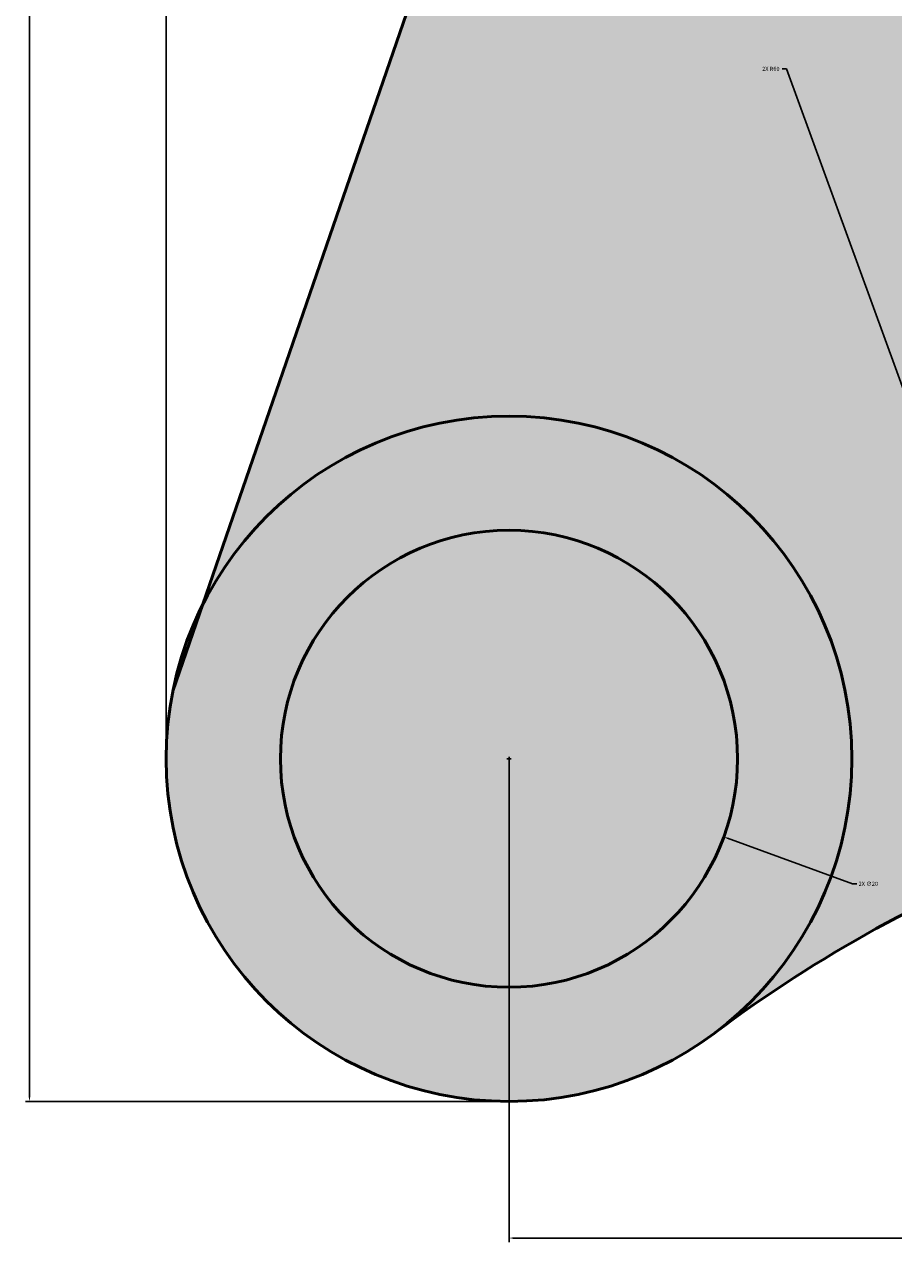
# Model space of a CAD drawing. Units: inches. Extents: x 114 to 236, y -51 to 115.
# Tile 2 of 14: x 114 to 152, y -13 to 41. Entities that reach past the tile are written whole.
import ezdxf

# ---------------------------------------------------------------- set-up
doc = ezdxf.new("R2010")
doc.units = ezdxf.units.IN
doc.header["$MEASUREMENT"] = 0
doc.layers.add('M-DIMS', color=2, linetype='Continuous', lineweight=18)
doc.layers.add('M-OUTL', color=7, linetype='Continuous', lineweight=50)
doc.layers.add('M-HATC', color=7, linetype='Continuous', lineweight=18, true_color=0xffffff)
doc.styles.get("Standard").update_dxf_attribs({"font": 'arial.ttf'})
doc.dimstyles.get("Standard").update_dxf_attribs({"dimtxt": 0.18, "dimasz": 0.18, "dimexe": 0.18, "dimexo": 0.0625, "dimgap": 0.09, "dimtad": 0, "dimtih": 1, "dimtoh": 1, "dimdec": 4, "dimzin": 0, "dimdsep": 46, "dimtxsty": 'Standard', "dimcen": 0.09, "dimadec": 0, "dimazin": 0, "dimtfac": 1, "dimtdec": 4, "dimtofl": 0, "dimtmove": 0, "dimatfit": 3, "dimfxl": 1, "dimtolj": 1, "dimtzin": 0, "dimarcsym": 0})

# ---------------------------------------------------------------- blocks, each defined once
blk = doc.blocks.new('BOSS-OD30-ID20')
for radius in [15, 10]:
    blk.add_circle((0, 0), radius)
blk = doc.blocks.new('*D3')
at = {"layer": 'Defpoints', "color": 0, "transparency": 16777216}
for p in [(230.229, 115.287), (120.229, 9.307), (230.229, 9.307)]:
    blk.add_point(p, dxfattribs=at)
at = {"layer": 'M-DIMS', "color": 0, "lineweight": -2, "transparency": 16777216}
for p, q in [((120.229, 9.37), (120.229, 115.467)), ((120.409, 115.287), (174.949, 115.287)), ((230.049, 115.287), (175.509, 115.287)), ((230.229, 9.37), (230.229, 115.467))]:
    blk.add_line(p, q, dxfattribs=at)
at = {"layer": 'M-DIMS', "color": 0, "transparency": 16777216}
for points in [[(120.409, 115.317), (120.409, 115.257), (120.229, 115.287)], [(230.049, 115.317), (230.049, 115.257), (230.229, 115.287)]]:
    blk.add_solid(points, dxfattribs=at)
at = {"layer": 'M-DIMS', "color": 0, "transparency": 16777216, "insert": (175.229, 115.287), "char_height": 0.18, "attachment_point": 5}
blk.add_mtext('\\A1;110', dxfattribs=at)
blk = doc.blocks.new('*D4')
at = {"layer": 'Defpoints', "color": 0, "transparency": 16777216}
for p in [(114.249, 109.307), (175.229, 109.307), (135.229, -5.693)]:
    blk.add_point(p, dxfattribs=at)
at = {"layer": 'M-DIMS', "color": 0, "lineweight": -2, "transparency": 16777216}
for p, q in [((175.166, 109.307), (114.069, 109.307)), ((114.249, 109.127), (114.249, 51.989)), ((114.249, -5.513), (114.249, 51.625)), ((135.166, -5.693), (114.069, -5.693))]:
    blk.add_line(p, q, dxfattribs=at)
at = {"layer": 'M-DIMS', "color": 0, "transparency": 16777216}
for points in [[(114.219, 109.127), (114.279, 109.127), (114.249, 109.307)], [(114.219, -5.513), (114.279, -5.513), (114.249, -5.693)]]:
    blk.add_solid(points, dxfattribs=at)
at = {"layer": 'M-DIMS', "color": 0, "transparency": 16777216, "insert": (114.249, 51.807), "char_height": 0.18, "attachment_point": 5}
blk.add_mtext('\\A1;115', dxfattribs=at)
blk = doc.blocks.new('*D5')
at = {"layer": 'Defpoints', "color": 0, "transparency": 16777216}
for p in [(175.229, 79.307), (135.229, 9.307), (175.229, -11.673)]:
    blk.add_point(p, dxfattribs=at)
at = {"layer": 'M-DIMS', "color": 0, "lineweight": -2, "transparency": 16777216}
for p, q in [((175.229, 79.245), (175.229, -11.853)), ((135.229, 9.245), (135.229, -11.853)), ((135.409, -11.673), (155.006, -11.673)), ((175.049, -11.673), (155.451, -11.673))]:
    blk.add_line(p, q, dxfattribs=at)
at = {"layer": 'M-DIMS', "color": 0, "transparency": 16777216}
for points in [[(135.409, -11.643), (135.409, -11.703), (135.229, -11.673)], [(175.049, -11.643), (175.049, -11.703), (175.229, -11.673)]]:
    blk.add_solid(points, dxfattribs=at)
at = {"layer": 'M-DIMS', "color": 0, "transparency": 16777216, "insert": (155.229, -11.673), "char_height": 0.18, "attachment_point": 5}
blk.add_mtext('\\A1;40', dxfattribs=at)
blk = doc.blocks.new('*D13')
at = {"layer": 'Defpoints', "color": 0, "transparency": 16777216}
for p in [(125.832, 12.727), (144.626, 5.887)]:
    blk.add_point(p, dxfattribs=at)
at = {"layer": 'M-DIMS', "color": 0, "lineweight": -2, "transparency": 16777216}
for p, q in [((135.139, 9.307), (135.319, 9.307)), ((135.229, 9.217), (135.229, 9.397)), ((150.264, 3.835), (144.795, 5.825)), ((150.444, 3.835), (150.264, 3.835))]:
    blk.add_line(p, q, dxfattribs=at)
at = {"layer": 'M-DIMS', "color": 0, "transparency": 16777216}
blk.add_solid([(144.805, 5.853), (144.784, 5.797), (144.626, 5.887)], dxfattribs=at)
at = {"layer": 'M-DIMS', "color": 0, "transparency": 16777216, "insert": (150.95, 3.835), "char_height": 0.18, "attachment_point": 5}
blk.add_mtext('\\A1;2X ∅20', dxfattribs=at)
blk = doc.blocks.new('*D14')
at = {"layer": 'Defpoints', "color": 0, "transparency": 16777216}
for p in [(159.689, 5.682), (180.229, -50.693)]:
    blk.add_point(p, dxfattribs=at)
at = {"layer": 'M-DIMS', "color": 0, "lineweight": -2, "transparency": 16777216}
for p, q in [((147.185, 39.507), (147.365, 39.507)), ((147.365, 39.507), (159.627, 5.851)), ((180.139, -50.693), (180.319, -50.693)), ((180.229, -50.783), (180.229, -50.603))]:
    blk.add_line(p, q, dxfattribs=at)
at = {"layer": 'M-DIMS', "color": 0, "transparency": 16777216}
blk.add_solid([(159.655, 5.861), (159.599, 5.841), (159.689, 5.682)], dxfattribs=at)
at = {"layer": 'M-DIMS', "color": 0, "transparency": 16777216, "insert": (146.685, 39.507), "char_height": 0.18, "attachment_point": 5}
blk.add_mtext('\\A1;2X R60', dxfattribs=at)

msp = doc.modelspace()

# ---------------------------------------------------------------- hatches: boundary and pattern name
at = {"layer": 'M-HATC'}
h = msp.add_hatch(color=256, dxfattribs=at)
h.set_gradient(color1=(242, 103, 34), color2=(255, 255, 0), tint=1, name='INVSPHERICAL')
h.paths.add_polyline_path([(145.229, 79.307, -0.060651), (146.105, 86.505), (121.823, 16.038, -0.790743), (150.229, 9.307, -0.236068), (144.229, -2.693, -0.14094), (175.229, 9.098, -0.14094), (206.229, -2.693, -0.236068), (200.229, 9.307, -0.790743), (228.634, 16.038), (204.352, 86.505, -0.060651), (205.229, 79.307, -1)])
h = msp.add_hatch(color=256, dxfattribs=at)
h.set_gradient(color1=(19, 155, 72), color2=(255, 255, 0), tint=1, name='HEMISPHERICAL')
h.paths.add_polyline_path([(121.823, 16.038), (120.523, 12.263, 0.049631), (120.229, 9.307, 1), (150.229, 9.307, 0.790743)])
h.paths.add_polyline_path([(145.229, 9.307, -1), (125.229, 9.307, -1)], flags=16)
msp.add_hatch(color=256, dxfattribs=at).paths.add_polyline_path([(125.229, 9.307, 1), (145.229, 9.307, 1)])

# ---------------------------------------------------------------- linework, layer by layer
at = {"layer": 'M-OUTL'}
msp.add_line((120.523, 12.263), (147.853, 91.577), dxfattribs=at)
msp.add_arc((180.229, -50.693), 60, 94.78019, 126.8699, dxfattribs=at)

# ---------------------------------------------------------------- block references
msp.add_blockref('BOSS-OD30-ID20', (135.229, 9.307), dxfattribs=at)

# ---------------------------------------------------------------- dimensions: what is measured, and where the dimension line sits
at = {"layer": 'M-DIMS'}
for base, p1, p2, picture, middle in [((230.229, 115.287), (120.229, 9.307), (230.229, 9.307), '*D3', (175.229, 115.287)), ((175.229, -11.673), (135.229, 9.307), (175.229, 79.307), '*D5', (155.229, -11.673))]:
    dim = msp.add_linear_dim(base=base, p1=p1, p2=p2, dimstyle='Standard', override={"dimdec": 0, "dimlfac": 1, "dimrnd": 0, "dimzin": 0, "dimdsep": 46, "dimlunit": 2}, dxfattribs=at)
    dim.commit()
    dim.dimension.update_dxf_attribs({"geometry": picture, "text_midpoint": middle})
dim = msp.add_linear_dim(base=(114.249, 109.307), p1=(135.229, -5.693), p2=(175.229, 109.307), angle=90, dimstyle='Standard', override={"dimdec": 0, "dimlfac": 1, "dimrnd": 0, "dimzin": 0, "dimdsep": 46, "dimlunit": 2}, dxfattribs=at)
dim.commit()
dim.dimension.update_dxf_attribs({"geometry": '*D4', "text_midpoint": (114.249, 51.807)})
dim = msp.add_radius_dim(center=(180.229, -50.693), mpoint=(159.689, 5.682), text='2X <>', dimstyle='Standard', override={"dimdec": 0, "dimlfac": 1, "dimrnd": 0, "dimzin": 0, "dimdsep": 46, "dimlunit": 2}, dxfattribs=at)
dim.commit()
dim.dimension.update_dxf_attribs({"geometry": '*D14', "text_midpoint": (146.685, 39.507), "dimtype": 164})
dim = msp.add_diameter_dim_2p(p1=(125.832, 12.727), p2=(144.626, 5.887), text='2X <>', dimstyle='Standard', override={"dimdec": 0, "dimlfac": 1, "dimrnd": 0, "dimzin": 0, "dimdsep": 46, "dimlunit": 2}, dxfattribs=at)
dim.commit()
dim.dimension.update_dxf_attribs({"geometry": '*D13', "text_midpoint": (150.95, 3.835), "dimtype": 163})

doc.saveas('drawing.dxf')
